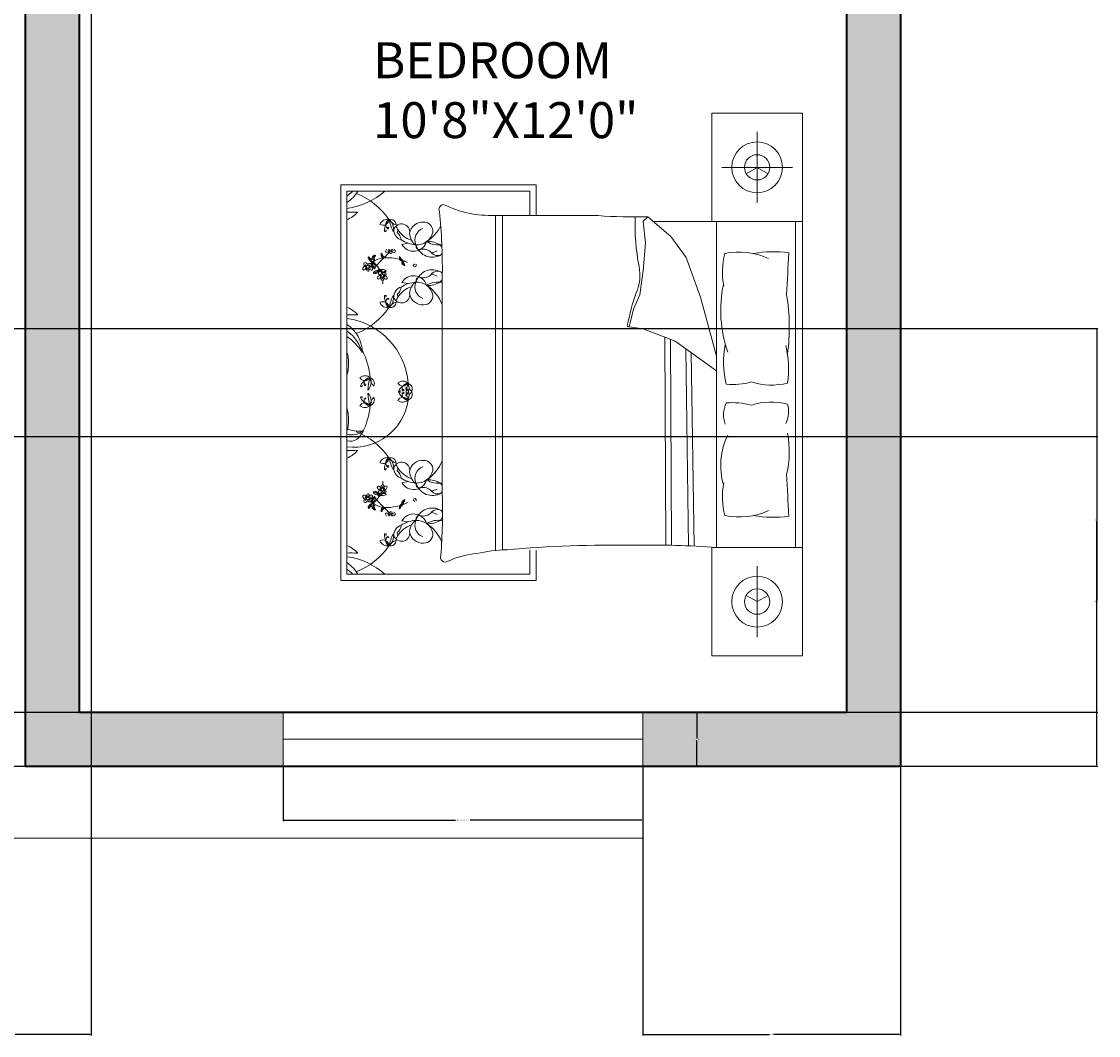
# Model space of a CAD drawing. Units: inches. Extents: x 37 to 706, y -568 to 110.
# Tile 16 of 24: x 526 to 706, y -568 to -398. Entities that reach past the tile are written whole.
import ezdxf

# ---------------------------------------------------------------- set-up
doc = ezdxf.new("R2010")
doc.units = ezdxf.units.IN
doc.header["$MEASUREMENT"] = 0
for name, color, linetype, lineweight in [('A-ANNO-DIMS', 2, 'Continuous', 18), ('A-AREA-IDEN', 7, 'Continuous', 18), ('A-FLOR-STRS', 7, 'Continuous', 18), ('A-FURN', 8, 'Continuous', 13), ('A-GLAZ', 4, 'Continuous', 18), ('A-WALL', 7, 'Continuous', 35), ('A-WALL-PATT', 252, 'Continuous', 13)]:
    doc.layers.add(name, color=color, linetype=linetype, lineweight=lineweight)
doc.styles.get("Standard").update_dxf_attribs({"font": 'arial.ttf'})
doc.dimstyles.get("Standard").update_dxf_attribs({"dimtxt": 0.18, "dimasz": 0.18, "dimexe": 0.18, "dimexo": 0.0625, "dimgap": 0.09, "dimtad": 0, "dimtih": 1, "dimtoh": 1, "dimdec": 0, "dimzin": 0, "dimdsep": 46, "dimlunit": 3, "dimtxsty": 'Standard', "dimcen": 0.09, "dimadec": 0, "dimazin": 0, "dimtfac": 1, "dimtdec": 0, "dimtofl": 0, "dimtmove": 0, "dimatfit": 3, "dimfxl": 1, "dimtolj": 1, "dimtzin": 0, "dimarcsym": 0})

# ---------------------------------------------------------------- blocks, each defined once
blk = doc.blocks.new('BED-DOUBLE-WITH-NIGHTSTANDS')
for p, q in [((77.02, 90.57), (77.02, 0)), ((69.47, 75.59), (69.47, 87.43)), ((63.56, 81.51), (75.39, 81.51)), ((0, 78.61), (32.62, 78.61)), ((0, 12.59), (0, 78.61)), ((1.05, 77.56), (1.05, 13.64)), ((31.58, 77.56), (1.05, 77.56)), ((31.58, 73.49), (31.58, 77.56)), ((32.62, 78.61), (32.62, 73.49)), ((25.85, 17.62), (25.85, 73.5)), ((26.98, 17.7), (26.98, 73.5)), ((50.48, 72.53), (51.22, 73.26)), ((50.85, 68.86), (50.48, 72.53)), ((51.22, 73.26), (55.07, 69.96)), ((77.02, 72.45), (52.16, 72.45)), ((62.71, 72.45), (62.71, 18.11)), ((75.86, 18.11), (75.86, 72.45)), ((10.23, 68.64), (11.25, 68.84)), ((50.48, 64.28), (50.85, 68.86)), ((55.07, 69.96), (57.63, 66.48)), ((57.63, 66.48), (60.02, 59.87)), ((16.95, 26.9), (16.95, 63.67)), ((49.93, 60.24), (50.48, 64.28)), ((10.23, 62.31), (11.25, 62.11)), ((48.83, 57.86), (49.93, 60.24)), ((60.02, 59.87), (62.71, 50)), ((48.1, 54.92), (48.83, 57.86)), ((50.48, 54.55), (48.1, 54.92)), ((55.8, 52.54), (50.48, 54.55)), ((54.24, 18.43), (54.09, 53.18)), ((55.17, 18.44), (55.03, 52.83)), ((62.71, 47.57), (55.8, 52.54)), ((58.02, 18.39), (57.55, 51.28)), ((58.95, 18.36), (58.49, 50.6)), ((10.23, 28.89), (11.25, 29.09)), ((10.23, 22.56), (11.25, 22.36)), ((31.58, 13.64), (31.58, 17.63)), ((32.62, 17.61), (32.62, 12.59)), ((69.47, 14.97), (69.47, 3.14)), ((32.62, 12.59), (0, 12.59)), ((1.05, 13.64), (31.58, 13.64))]:
    blk.add_line(p, q)
for points in [[(61.93, 72.45), (61.93, 90.57), (77.02, 90.57)], [(69.47, 81.51), (67.64, 80.45)], [(69.47, 81.51), (71.3, 80.45)], [(77.02, 18.11), (61.93, 18.11), (61.93, 0), (77.02, 0)], [(69.47, 9.06), (67.64, 10.11)], [(69.47, 9.06), (71.3, 10.11)]]:
    blk.add_lwpolyline(points)
for points in [[(42.92, 73.45, 0.001242), (25.74, 73.5, -0.127202), (17.18, 75.31)], [(74.76, 67.25, 0.074897), (68.85, 67.14, -0.472817)], [(68.52, 45.71, 0.14099), (74.55, 45.53, 0.235245)], [(68.52, 41.84, -0.14099), (74.55, 42.02, -0.235245)], [(74.76, 23.32, -0.074897), (68.85, 23.42, 0.472817)], [(27.69, 17.73, 0.056112), (22.71, 17.07, 0.095341), (17.91, 15.8)]]:
    blk.add_lwpolyline(points, format="xyb")
for centre, radius in [((69.47, 81.51), 4.23), ((69.47, 81.51), 2.11), ((4.52, 64.91), 0.231), ((6.95, 63.41), 0.231), ((6.95, 27.79), 0.231), ((4.52, 26.28), 0.231), ((69.47, 9.06), 4.23), ((69.47, 9.06), 2.11)]:
    blk.add_circle(centre, radius)
for centre, radius, start, end in [((-3.2, 82.51), 7.18, 306.3036, 316.4814), ((-2.13, 80.43), 5.76, 303.4617, 330.1116), ((-0.54, 86.37), 11.83, 277.745, 311.8856), ((-1.71, 66.13), 11.83, 34.3865, 68.5908), ((-0.79, 77.21), 4.81, 292.5547, 318.9546), ((1.79, 90.38), 16.36, 267.4081, 273.6519), ((17.23, 74.48), 0.836, 93.98, 207.3412), ((-77.32, 64.75), 94.28, 359.3433, 5.6887), ((7.77, 71.53), 1.31, 77.7115, 159.0387), ((7.06, 72.84), 0.988, 238.4633, 358.2869), ((10.3, 70.85), 2.99, 138.8402, 177.9352), ((8.5, 71.96), 0.967, 117.6827, 223.7762), ((8.28, 71.86), 0.98, 2.9516, 103.728), ((16.12, 74.61), 8.27, 192.5173, 207.1824), ((6.95, 71.3), 1.87, 345.4653, 54.2343), ((9.77, 73.87), 2.02, 211.3827, 255.2969), ((10.16, 70.71), 1.36, 350.264, 160.8688), ((13.65, 70.21), 2.16, 84.9449, 172.8857), ((13.86, 70.84), 1.53, 354.4856, 91.0538), ((48.97, 156.3), 83.07, 265.8294, 271.553), ((83.29, 71.71), 34.18, 177.4519, 191.3392), ((7.46, 70.95), 0.147, 177.9352, 11.4834), ((7.53, 70.96), 0.0713, 11.4834, 127.9409), ((7.89, 71.38), 0.128, 223.7762, 159.7183), ((10.57, 71.04), 1.7, 175.969, 254.3045), ((8.69, 70.99), 0.833, 333.9755, 53.2681), ((8.31, 69.21), 1.81, 6.1662, 51.5825), ((13.15, 73.4), 4.28, 211.2614, 251.7045), ((14.13, 70.59), 2.63, 182.3591, 234.0401), ((14.47, 69.36), 2.1, 111.5819, 201.4221), ((12.73, 71.31), 2.72, 265.2933, 346.921), ((10.57, 74.83), 6.85, 303.6671, 333.2997), ((12.81, 73.44), 4.86, 236.2883, 266.5076), ((12.18, 69.76), 2.25, 209.9085, 343.1337), ((13.13, 68.34), 0.562, 167.3041, 285.1471), ((14.65, 65.65), 3.49, 122.7011, 126.3445), ((15.31, 69.41), 2.89, 199.2822, 299.1751), ((16.28, 72.32), 3.75, 238.8218, 279.1554), ((14.65, 65.65), 3.49, 55.785, 94.7304), ((15.95, 67.67), 1.09, 30.0293, 52.325), ((4.85, 66.4), 0.258, 124.3538, 214.3923), ((5.41, 66.58), 0.697, 176.9701, 248.2913), ((10.38, 70.25), 6.74, 212.6784, 216.3746), ((5.81, 66.23), 0.6, 122.8155, 187.3992), ((6.07, 66.15), 0.697, 109.4799, 177.6828), ((5.7, 66.59), 0.258, 56.8636, 146.9021), ((11.37, 62.96), 6.74, 145.1882, 148.8844), ((9.29, 67.11), 2.55, 178.3264, 187.1302), ((6.53, 66.75), 0.476, 11.3256, 64.4621), ((8.15, 67.44), 1.43, 190.2588, 210.656), ((7.19, 66.85), 0.435, 188.3432, 274.2869), ((7.57, 67.09), 0.759, 210.656, 242.6341), ((8.14, 67.75), 1.46, 218.2101, 226.3071), ((7.07, 66.52), 0.185, 325.7657, 67.4417), ((1.34, 72.69), 8.6, 313.1541, 322.0459), ((7.66, 67.53), 0.177, 142.4737, 265.053), ((7.89, 67.56), 0.381, 127.7621, 169.0403), ((7.69, 67.89), 0.536, 265.053, 338.3618), ((8.4, 67.15), 0.7, 113.4276, 137.6104), ((8.32, 67.88), 0.231, 183.2768, 356.7232), ((8.49, 67.46), 0.377, 139.7889, 227.6792), ((8.37, 67.33), 0.199, 227.6792, 350.3487), ((7.6, 67.46), 0.755, 353.0852, 15.7171), ((8.1, 67.37), 0.477, 350.3487, 43.6538), ((8.98, 67.87), 0.555, 198.7263, 262.5032), ((8.54, 67.61), 0.22, 1.1081, 91.8675), ((8.68, 67.56), 0.385, 11.5637, 52.6358), ((8.95, 67.49), 0.178, 255.2356, 54.9248), ((12.34, 66.57), 2.55, 178.3264, 187.1302), ((9.58, 66.21), 0.476, 11.3256, 64.4621), ((11.19, 66.9), 1.43, 190.2588, 210.656), ((13.76, 66), 1.86, 41.5653, 105.1471), ((14.78, 69.85), 2.6, 277.436, 299.9149), ((16.16, 68.13), 1.36, 221.5653, 293.8354), ((15.95, 67.67), 1.09, 314.4517, 333.558), ((75.82, 64.02), 12.14, 165.1039, 191.0369), ((66.47, 55.71), 11.67, 65.1316, 101.7583), ((936.66, 17.33), 863.34, 176.68521, 177.14978), ((3.86, 64.56), 0.177, 142.4737, 265.053), ((4.09, 64.6), 0.381, 61.2196, 169.0403), ((3.89, 64.92), 0.536, 265.053, 338.3618), ((4.34, 65.38), 0.455, 157.4086, 261.4386), ((4.09, 65.4), 0.229, 58.0499, 135.6268), ((4.6, 64.19), 0.7, 113.4276, 137.6104), ((4.32, 65.26), 0.153, 172.906, 277.132), ((3.82, 64.98), 0.727, 14.7558, 58.0499), ((4.69, 64.5), 0.377, 139.7889, 227.6792), ((4.84, 65.17), 0.315, 36.1046, 181.4281), ((3.8, 64.5), 0.755, 353.0852, 15.7171), ((5.23, 66.36), 0.6, 190.3057, 287.1958), ((4.29, 64.41), 0.477, 350.3487, 43.6538), ((5.18, 64.9), 0.555, 198.7263, 262.5032), ((4.66, 65.42), 0.317, 270.0645, 331.1507), ((4.93, 65.34), 0.363, 221.8413, 265.7877), ((4.74, 64.65), 0.22, 1.1081, 91.8675), ((4.92, 65.2), 0.226, 263.7526, 41.7054), ((4.88, 64.6), 0.385, 11.5637, 86.365), ((5.17, 66.41), 0.267, 216.3746, 291.7548), ((7.53, 62.67), 3.76, 124.0033, 132.4917), ((5.15, 64.53), 0.178, 255.2356, 54.9248), ((3.66, 62.2), 4.02, 63.7819, 68.2913), ((5.81, 65.29), 0.639, 128.3208, 208.8162), ((5.92, 65.34), 0.764, 207.7043, 254.3516), ((5.34, 65.98), 0.201, 289.3605, 111.7548), ((5.49, 65.98), 0.201, 221.8703, 44.2646), ((6.41, 65.39), 1.05, 157.2305, 229.0635), ((6.05, 65.74), 0.619, 174.4544, 220.6188), ((2.53, 62.29), 4.51, 30.544, 49.818), ((5.83, 66.31), 0.267, 148.8844, 224.2646), ((5.02, 64.86), 0.744, 340.0041, 40.6188), ((7.53, 62.67), 3.76, 94.756, 119.2041), ((15.54, 57.26), 12.37, 132.2412, 142.1744), ((7.72, 58.94), 7.5, 73.5842, 93.8277), ((10.23, 66.31), 0.435, 188.3432, 274.2869), ((10.61, 66.55), 0.759, 210.656, 242.6341), ((11.19, 67.21), 1.46, 218.2101, 226.3071), ((10.11, 65.98), 0.185, 325.7657, 67.4417), ((10.63, 65.65), 0.435, 147.5332, 233.4768), ((11.02, 65.87), 0.759, 179.1859, 211.164), ((10.28, 65.7), 0.185, 354.3784, 96.0543), ((7.72, 58.94), 7.5, 63.0032, 69.8941), ((11.6, 66.22), 1.43, 211.164, 231.5612), ((11.85, 67.38), 2.55, 234.6898, 243.4936), ((11.87, 66.07), 1.46, 195.5129, 203.6099), ((10.23, 65.12), 0.476, 357.3579, 50.4944), ((12.28, 65.21), 0.175, 12.7051, 190.4384), ((12.38, 65.23), 0.284, 190.4384, 10.4136), ((42.55, 63.54), 7.37, 336.2616, 11.3392), ((4.57, 64.37), 0.199, 227.6792, 350.3487), ((5.43, 64.9), 1.05, 270.278, 342.111), ((6.13, 63.58), 0.744, 98.7227, 159.3375), ((5.75, 64.54), 0.764, 244.9899, 291.6373), ((5.92, 64.93), 0.619, 278.7227, 324.8872), ((5.81, 64.43), 0.639, 290.5253, 358.5375), ((6.29, 63.06), 0.177, 142.4737, 265.053), ((6.52, 63.09), 0.381, 61.2196, 169.0403), ((6.32, 63.41), 0.536, 265.053, 338.3618), ((6.77, 63.88), 0.455, 157.4086, 261.4386), ((6.52, 63.89), 0.229, 58.0499, 135.6268), ((7.06, 64.61), 0.639, 182.8499, 266.1226), ((6.81, 65.06), 0.619, 231.7607, 277.9252), ((7.29, 65.17), 1.05, 214.5369, 286.3699), ((7.03, 62.68), 0.7, 113.4276, 137.6104), ((6.76, 63.75), 0.153, 172.906, 277.132), ((6.25, 63.47), 0.727, 14.7558, 58.0499), ((2.53, 62.29), 4.51, 23.0501, 23.8477), ((7.12, 62.99), 0.377, 139.7889, 227.6792), ((7, 63.71), 0.744, 37.3105, 97.9252), ((7.27, 63.66), 0.315, 36.1046, 181.4281), ((6.23, 62.99), 0.755, 353.0852, 15.7171), ((7.08, 64.73), 0.764, 265.0106, 311.658), ((6.72, 62.9), 0.477, 350.3487, 43.6538), ((7.61, 63.4), 0.555, 198.7263, 262.5032), ((7.09, 63.91), 0.317, 270.0645, 331.1507), ((7.36, 63.83), 0.363, 221.8413, 265.7877), ((7.17, 63.14), 0.22, 1.1081, 91.8675), ((7.36, 63.7), 0.226, 263.7526, 41.7054), ((7.31, 63.09), 0.385, 11.5637, 86.365), ((7.58, 63.02), 0.178, 255.2356, 54.9248), ((12.18, 61.19), 2.25, 16.8663, 150.0915), ((13.13, 62.61), 0.562, 74.8529, 192.6959), ((15.31, 61.54), 2.89, 60.8249, 160.7178), ((13.76, 64.95), 1.86, 254.8529, 318.4347), ((14.78, 61.1), 2.6, 60.0851, 82.564), ((16.16, 62.82), 1.36, 66.1646, 138.4347), ((15.95, 63.28), 1.09, 23.229, 45.5483), ((7, 62.86), 0.199, 227.6792, 350.3487), ((2.53, 62.29), 4.51, 357.1071, 4.7585), ((10.57, 59.91), 1.7, 105.6955, 184.031), ((8.31, 61.74), 1.81, 308.4175, 353.8338), ((13.15, 57.54), 4.28, 108.2955, 148.7386), ((12.81, 57.5), 4.86, 93.4924, 123.7117), ((14.13, 60.36), 2.63, 125.9599, 177.6409), ((14.47, 61.59), 2.1, 158.5779, 248.4181), ((12.73, 59.64), 2.72, 13.079, 94.7067), ((14.65, 65.3), 3.49, 233.6555, 237.2989), ((16.28, 58.63), 3.75, 79.7133, 121.1782), ((14.65, 65.3), 3.49, 265.2696, 304.215), ((10.57, 56.11), 6.85, 21.4941, 56.3329), ((15.95, 63.28), 1.09, 307.675, 336.7144), ((84.45, 57.63), 21.05, 168.0397, 199.2615), ((7.46, 60), 0.147, 348.5166, 182.0648), ((10.3, 60.1), 2.99, 182.0648, 221.1598), ((7.53, 59.98), 0.0713, 232.0591, 348.5166), ((8.5, 58.99), 0.967, 136.2238, 242.3173), ((7.94, 59.56), 0.0771, 200.2667, 136.2271), ((6.95, 59.65), 1.87, 305.7657, 14.5347), ((16.12, 56.34), 8.27, 152.8176, 167.4827), ((10.16, 60.24), 1.36, 199.1312, 9.736), ((8.69, 59.96), 0.833, 306.7319, 26.0245), ((13.65, 60.74), 2.16, 187.1143, 275.0551), ((13.86, 60.11), 1.53, 268.9462, 5.5144), ((82.33, 48.63), 35.12, 160.1194, 169.3383), ((41.99, 54.84), 32.85, 352.2196, 9.497), ((-0.79, 53.74), 4.81, 41.0454, 67.4453), ((-1.71, 64.81), 11.83, 291.4092, 325.6135), ((7.06, 58.1), 0.988, 1.7131, 121.5367), ((7.77, 59.41), 1.31, 200.9613, 282.2885), ((8.28, 59.09), 0.98, 256.272, 357.0484), ((9.77, 57.08), 2.02, 104.7031, 148.6173), ((1.79, 40.57), 16.36, 86.3481, 92.5919), ((-0.54, 44.58), 11.83, 4.4623, 82.255), ((-2.13, 50.51), 5.76, 1.272, 56.5383), ((-3.2, 48.44), 7.18, 17.8504, 53.6964), ((48.03, 55.13), 0.219, 178.8623, 289.7536), ((-5.22, 44.66), 10.68, 34.0123, 54.053), ((-5.17, 48.79), 6.5, 343.5431, 17.0202), ((-6.88, 45.48), 11.83, 4.4623, 27.4146), ((79.85, 49.11), 15.97, 169.8617, 193.6238), ((58.59, 47.9), 16.14, 351.5249, 13.96), ((-8.52, 46.22), 9.62, 4.3787, 5.6357), ((-15.11, 41.15), 17.18, 19.7217, 19.9028), ((4.03, 45.43), 1.31, 47.7873, 129.1145), ((4.07, 46.92), 0.988, 208.5391, 328.3627), ((3.47, 45.08), 0.147, 148.011, 341.5592), ((5.88, 43.58), 2.99, 108.9159, 148.011), ((3.54, 45.06), 0.0713, 341.5592, 98.0167), ((4.87, 45.44), 0.967, 87.7585, 193.852), ((4.06, 45.24), 0.128, 193.852, 129.9245), ((12.81, 43.93), 8.27, 162.593, 177.2582), ((3.21, 45.64), 1.87, 315.5411, 24.3101), ((6.93, 46.46), 2.02, 181.4585, 225.3727), ((4.64, 45.46), 0.98, 333.0274, 73.8037), ((10.37, 44.53), 1.31, 47.7873, 129.1145), ((10.41, 46.02), 0.988, 208.5391, 328.3627), ((12.22, 42.67), 2.99, 108.9159, 148.011), ((11.21, 44.53), 0.967, 87.7585, 193.852), ((9.54, 44.73), 1.87, 315.5411, 24.3101), ((19.14, 43.02), 8.27, 162.593, 177.2582), ((10.97, 44.56), 0.98, 333.0274, 73.8037), ((13.27, 45.55), 2.02, 181.4585, 225.3727), ((65.49, 56.38), 11.1, 264.0129, 285.8293), ((3.47, 43.1), 0.147, 18.4408, 211.989), ((3.54, 43.12), 0.0713, 261.9833, 18.4408), ((12.81, 44.25), 8.27, 182.7418, 197.407), ((3.21, 42.54), 1.87, 335.6899, 44.4589), ((6.93, 41.72), 2.02, 134.6273, 178.5415), ((4.64, 42.72), 0.98, 286.1963, 26.9726), ((10.41, 42.16), 0.988, 31.6373, 151.4609), ((9.8, 44.18), 0.147, 148.011, 341.5592), ((9.8, 44), 0.147, 18.4408, 211.989), ((12.22, 45.51), 2.99, 211.989, 251.0841), ((9.88, 44.15), 0.0713, 341.5592, 98.0167), ((9.88, 44.03), 0.0713, 261.9833, 18.4408), ((11.21, 43.65), 0.967, 166.148, 272.2415), ((10.39, 44.33), 0.128, 193.852, 129.9245), ((10.44, 43.86), 0.0771, 230.1909, 166.0209), ((9.54, 43.45), 1.87, 335.6899, 44.4589), ((19.14, 45.16), 8.27, 182.7418, 197.407), ((10.97, 43.62), 0.98, 286.1963, 26.9726), ((13.27, 42.63), 2.02, 134.6273, 178.5415), ((2.19, 43.98), 9.15, 262.8636, 351.8197), ((4.07, 41.26), 0.988, 31.6373, 151.4609), ((4.03, 42.75), 1.31, 230.8855, 312.2127), ((5.88, 44.6), 2.99, 211.989, 251.0841), ((-6.88, 42.69), 11.83, 332.5854, 355.5377), ((4.87, 42.74), 0.967, 166.148, 272.2415), ((4.11, 42.95), 0.0771, 230.1909, 166.0209), ((10.37, 43.65), 1.31, 230.8855, 312.2127), ((68.68, 40.17), 4.8, 155.0183, 198.5407), ((65.49, 31.16), 11.1, 74.1707, 95.9871), ((70.25, 40.78), 4.48, 333.3437, 16.1026), ((-5.17, 39.39), 6.5, 342.9798, 16.4569), ((-8.52, 41.96), 9.62, 354.3643, 355.6213), ((-15.11, 47.03), 17.18, 340.0972, 340.2783), ((3.02, 42.8), 5.3, 248.117, 276.6195), ((1.55, 37.94), 2.12, 256.3898, 349.0739), ((1.84, 39.54), 2.68, 252.8609, 311.9049), ((-1.71, 26.39), 11.83, 34.3865, 68.5908), ((74.93, 31.78), 11.53, 153.8761, 196.1746), ((58.92, 34.06), 15.92, 346.3427, 11.1841), ((1.79, 50.63), 16.36, 267.4081, 273.6519), ((-0.79, 37.46), 4.81, 292.5547, 318.9546), ((7.77, 31.78), 1.31, 77.7115, 159.0387), ((7.06, 33.09), 0.988, 238.4633, 358.2869), ((10.3, 31.1), 2.99, 138.8402, 177.9352), ((8.5, 32.21), 0.967, 117.6827, 223.7762), ((8.28, 32.11), 0.98, 2.9516, 103.728), ((9.77, 34.12), 2.02, 211.3827, 255.2969), ((6.95, 31.55), 1.87, 345.4653, 54.2343), ((16.12, 34.86), 8.27, 192.5173, 207.1824), ((13.65, 30.46), 2.16, 84.9449, 172.8857), ((13.86, 31.09), 1.53, 354.4856, 91.0538), ((10.57, 35.08), 6.85, 303.6671, 338.5059), ((7.46, 31.2), 0.147, 177.9352, 11.4834), ((7.53, 31.21), 0.0713, 11.4834, 127.9409), ((7.89, 31.63), 0.128, 223.7762, 159.7183), ((10.16, 30.96), 1.36, 350.264, 160.8688), ((10.57, 31.29), 1.7, 175.969, 254.3045), ((8.69, 31.24), 0.833, 333.9755, 53.2681), ((8.31, 29.46), 1.81, 6.1662, 51.5825), ((13.15, 33.66), 4.28, 211.2614, 251.7045), ((14.13, 30.84), 2.63, 182.3591, 234.0401), ((14.47, 29.61), 2.1, 111.5819, 201.4221), ((12.73, 31.56), 2.72, 265.2933, 346.921), ((2.53, 28.91), 4.51, 355.2415, 2.8929), ((12.81, 33.7), 4.86, 236.2883, 266.5076), ((12.18, 30.01), 2.25, 209.9085, 343.1337), ((14.65, 25.9), 3.49, 122.7011, 126.3445), ((16.28, 32.57), 3.75, 238.8218, 280.2867), ((14.65, 25.9), 3.49, 55.785, 94.7304), ((15.95, 27.92), 1.09, 23.2856, 52.325), ((75.82, 26.55), 12.14, 168.9631, 194.8961), ((936.66, 73.23), 863.34, 182.85022, 183.31479), ((4.69, 26.7), 0.377, 132.3208, 220.2111), ((4.57, 26.83), 0.199, 9.6513, 132.3208), ((5.75, 26.66), 0.764, 68.3627, 115.0101), ((5.43, 26.3), 1.05, 17.889, 89.722), ((6.13, 27.61), 0.744, 200.6625, 261.2773), ((5.81, 26.77), 0.639, 1.4625, 69.4747), ((6.29, 28.14), 0.177, 94.947, 217.5263), ((6.52, 28.11), 0.381, 190.9597, 298.7804), ((6.32, 27.78), 0.536, 21.6382, 94.947), ((6.77, 27.32), 0.455, 98.5614, 202.5914), ((6.52, 27.31), 0.229, 224.3732, 301.9501), ((7.06, 26.59), 0.639, 93.8774, 177.1501), ((7.29, 26.03), 1.05, 73.6301, 145.4631), ((7.03, 28.52), 0.7, 222.3896, 246.5724), ((6.76, 27.45), 0.153, 82.868, 187.094), ((6.25, 27.73), 0.727, 301.9501, 345.2442), ((2.53, 28.91), 4.51, 336.1523, 336.9499), ((7.12, 28.21), 0.377, 132.3208, 220.2111), ((7, 28.34), 0.199, 9.6513, 132.3208), ((7, 27.49), 0.744, 262.0748, 322.6895), ((6.23, 28.2), 0.755, 344.2829, 6.9148), ((7.27, 27.54), 0.315, 178.5719, 323.8954), ((7.08, 26.46), 0.764, 48.342, 94.9894), ((6.72, 28.3), 0.477, 316.3462, 9.6513), ((7.61, 27.8), 0.555, 97.4968, 161.2737), ((7.36, 27.37), 0.363, 94.2123, 138.1587), ((7.09, 27.29), 0.317, 28.8493, 89.9355), ((7.17, 28.06), 0.22, 268.1325, 358.8919), ((7.31, 28.11), 0.385, 273.635, 348.4363), ((7.36, 27.5), 0.226, 318.2946, 96.2474), ((7.58, 28.18), 0.178, 305.0752, 104.7644), ((13.13, 28.59), 0.562, 167.3041, 285.1471), ((15.31, 29.66), 2.89, 199.2822, 299.1751), ((13.76, 26.25), 1.86, 41.5653, 105.1471), ((14.78, 30.1), 2.6, 277.436, 299.9149), ((16.16, 28.38), 1.36, 221.5653, 293.8354), ((15.95, 27.92), 1.09, 314.4517, 336.7144), ((3.86, 26.63), 0.177, 94.947, 217.5263), ((4.09, 26.6), 0.381, 190.9597, 298.7804), ((3.89, 26.28), 0.536, 21.6382, 94.947), ((4.34, 25.81), 0.455, 98.5614, 202.5914), ((4.09, 25.8), 0.229, 224.3732, 301.9501), ((4.6, 27.01), 0.7, 222.3896, 246.5724), ((4.32, 25.94), 0.153, 82.868, 187.094), ((3.82, 26.22), 0.727, 301.9501, 345.2442), ((4.84, 26.03), 0.315, 178.5719, 323.8954), ((3.8, 26.7), 0.755, 344.2829, 6.9148), ((4.29, 26.79), 0.477, 316.3462, 9.6513), ((5.23, 24.83), 0.6, 72.8042, 169.6943), ((5.18, 26.29), 0.555, 97.4968, 161.2737), ((4.93, 25.86), 0.363, 94.2123, 138.1587), ((4.66, 25.78), 0.317, 28.8493, 89.9355), ((5.41, 24.62), 0.697, 111.7087, 183.0299), ((4.74, 26.55), 0.22, 268.1325, 358.8919), ((4.88, 26.6), 0.385, 273.635, 348.4363), ((4.92, 25.99), 0.226, 318.2946, 96.2474), ((7.53, 28.53), 3.76, 227.5083, 235.9967), ((5.15, 26.67), 0.178, 305.0752, 104.7644), ((3.66, 29), 4.02, 291.7087, 296.2181), ((5.81, 25.91), 0.639, 151.1838, 231.6792), ((5.92, 25.86), 0.764, 105.6484, 152.2957), ((5.34, 25.22), 0.201, 248.2452, 70.6395), ((6.41, 25.8), 1.05, 130.9365, 202.7695), ((5.49, 25.22), 0.201, 315.7354, 138.1297), ((6.05, 25.46), 0.619, 139.3812, 185.5456), ((2.53, 28.91), 4.51, 310.182, 329.456), ((5.02, 26.34), 0.744, 319.3812, 19.9959), ((7.53, 28.53), 3.76, 240.7959, 265.244), ((15.54, 33.94), 12.37, 217.8256, 227.7588), ((5.92, 26.27), 0.619, 35.1128, 81.2773), ((6.81, 26.14), 0.619, 82.0748, 128.2393), ((10.23, 24.88), 0.435, 85.7131, 171.6568), ((10.61, 24.64), 0.759, 117.3659, 149.344), ((10.11, 25.21), 0.185, 292.5583, 34.2343), ((10.63, 25.55), 0.435, 126.5232, 212.4668), ((11.02, 25.33), 0.759, 148.836, 180.8141), ((10.28, 25.5), 0.185, 263.9457, 5.6216), ((7.72, 32.26), 7.5, 290.1059, 296.9968), ((11.6, 24.98), 1.43, 128.4388, 148.836), ((11.85, 23.82), 2.55, 116.5064, 125.3102), ((11.87, 25.13), 1.46, 156.3901, 164.4871), ((10.23, 26.08), 0.476, 309.5056, 2.6421), ((12.28, 25.98), 0.175, 169.5616, 347.2949), ((12.38, 25.96), 0.284, 349.5864, 169.5616), ((-71.13, 24.12), 88.13, 355.2402, 1.8035), ((4.85, 24.8), 0.258, 145.6077, 235.6462), ((10.38, 20.95), 6.74, 143.6254, 147.3216), ((5.17, 24.78), 0.267, 68.2452, 143.6254), ((5.81, 24.97), 0.6, 172.6008, 237.1845), ((6.07, 25.05), 0.697, 182.3172, 250.5201), ((5.7, 24.61), 0.258, 213.0979, 303.1364), ((5.83, 24.89), 0.267, 135.7354, 211.1156), ((11.37, 28.24), 6.74, 211.1156, 214.8118), ((8.15, 23.76), 1.43, 149.344, 169.7412), ((9.29, 24.09), 2.55, 172.8698, 181.6736), ((6.53, 24.45), 0.476, 295.5379, 348.6744), ((7.19, 24.34), 0.435, 85.7131, 171.6568), ((7.57, 24.1), 0.759, 117.3659, 149.344), ((8.14, 23.45), 1.46, 133.6929, 141.7899), ((7.07, 24.67), 0.185, 292.5583, 34.2343), ((7.72, 32.26), 7.5, 266.1723, 286.4158), ((1.34, 18.5), 8.6, 37.9541, 46.8459), ((7.66, 23.67), 0.177, 94.947, 217.5263), ((7.89, 23.64), 0.381, 190.9597, 232.2379), ((7.69, 23.31), 0.536, 21.6382, 94.947), ((8.4, 24.05), 0.7, 222.3896, 246.5724), ((8.32, 23.32), 0.231, 3.2768, 176.7232), ((8.49, 23.74), 0.377, 132.3208, 220.2111), ((8.37, 23.87), 0.199, 9.6513, 132.3208), ((7.6, 23.73), 0.755, 344.2829, 6.9148), ((8.1, 23.82), 0.477, 316.3462, 9.6513), ((8.98, 23.33), 0.555, 97.4968, 161.2737), ((8.54, 23.59), 0.22, 268.1325, 358.8919), ((8.95, 23.71), 0.178, 305.0752, 104.7644), ((8.68, 23.64), 0.385, 307.3642, 348.4363), ((11.19, 24.3), 1.43, 149.344, 169.7412), ((12.34, 24.63), 2.55, 172.8698, 181.6736), ((9.58, 24.98), 0.476, 295.5379, 348.6744), ((11.19, 23.99), 1.46, 133.6929, 141.7899), ((12.18, 21.44), 2.25, 16.8663, 150.0915), ((13.13, 22.86), 0.562, 74.8529, 192.6959), ((15.31, 21.79), 2.89, 60.8249, 160.7178), ((13.76, 25.2), 1.86, 254.8529, 318.4347), ((14.78, 21.35), 2.6, 60.0851, 82.564), ((16.16, 23.07), 1.36, 66.1646, 138.4347), ((15.95, 23.53), 1.09, 16.6343, 45.5483), ((66.47, 34.85), 11.67, 258.2417, 294.8684), ((10.57, 20.16), 1.7, 105.6955, 184.031), ((8.31, 21.99), 1.81, 308.4175, 353.8338), ((13.15, 17.79), 4.28, 108.2955, 148.7386), ((12.81, 17.75), 4.86, 93.4924, 123.7117), ((14.13, 20.61), 2.63, 125.9599, 177.6409), ((14.47, 21.84), 2.1, 158.5779, 248.4181), ((12.73, 19.89), 2.72, 13.079, 94.7067), ((14.65, 25.55), 3.49, 233.6555, 237.2989), ((16.28, 18.88), 3.75, 79.249, 121.1782), ((14.65, 25.55), 3.49, 265.2696, 304.215), ((10.57, 16.37), 6.85, 23.6453, 56.3329), ((15.95, 23.53), 1.09, 307.675, 342.5814), ((7.46, 20.25), 0.147, 348.5166, 182.0648), ((10.3, 20.35), 2.99, 182.0648, 221.1598), ((7.53, 20.24), 0.0713, 232.0591, 348.5166), ((8.5, 19.24), 0.967, 136.2238, 242.3173), ((7.94, 19.81), 0.0771, 200.2667, 136.2271), ((16.12, 16.59), 8.27, 152.8176, 167.4827), ((6.95, 19.9), 1.87, 305.7657, 14.5347), ((10.16, 20.49), 1.36, 199.1312, 9.736), ((8.69, 20.21), 0.833, 306.7319, 26.0245), ((13.65, 20.99), 2.16, 187.1143, 275.0551), ((13.86, 20.36), 1.53, 268.9462, 5.5144), ((-0.79, 13.99), 4.81, 41.0454, 67.4453), ((-1.71, 25.06), 11.83, 291.4092, 325.6135), ((7.06, 18.36), 0.988, 1.7131, 121.5367), ((7.77, 19.67), 1.31, 200.9613, 282.2885), ((9.77, 17.33), 2.02, 104.7031, 148.6173), ((8.28, 19.34), 0.98, 256.272, 357.0484), ((45.72, -193.78), 212.28, 89.1145, 94.8735), ((51.64, -144.24), 162.73, 86.1, 90.9282), ((1.79, 0.82), 16.36, 86.3481, 92.5919), ((-0.54, 4.83), 11.83, 48.1144, 82.255), ((17.45, 16.48), 0.826, 156.5219, 303.8264), ((-2.13, 10.76), 5.76, 29.8884, 56.5383), ((-3.2, 8.69), 7.18, 43.5186, 53.6964)]:
    blk.add_arc(centre, radius, start, end)
blk = doc.blocks.new('WIN-60')
for p, q in [((60, 9), (0, 9)), ((0, 9), (0, 0)), ((60, 0), (60, 9)), ((60, 4.5), (0, 4.5)), ((0, 0), (60, 0))]:
    blk.add_line(p, q)
blk = doc.blocks.new('ENTRY-STEP-236')
for p, q in [((236, 12), (236, 0)), ((236, 0), (0, 0))]:
    blk.add_line(p, q)
blk = doc.blocks.new('*D19')
at = {"layer": 'A-ANNO-DIMS', "color": 0, "lineweight": -2, "transparency": 16777216}
for p, q in [((569.96, -522.77), (569.96, -531.89)), ((629.96, -522.77), (629.96, -531.89)), ((570.14, -531.71), (598.73, -531.71)), ((629.78, -531.71), (601.19, -531.71))]:
    blk.add_line(p, q, dxfattribs=at)
at = {"layer": 'A-ANNO-DIMS', "color": 0, "transparency": 16777216}
for points in [[(570.14, -531.68), (570.14, -531.74), (569.96, -531.71)], [(629.78, -531.68), (629.78, -531.74), (629.96, -531.71)]]:
    blk.add_solid(points, dxfattribs=at)
at = {"layer": 'Defpoints', "color": 0, "transparency": 16777216}
for p in [(569.96, -522.71), (629.96, -522.71), (629.96, -531.71)]:
    blk.add_point(p, dxfattribs=at)
at = {"layer": 'A-ANNO-DIMS', "color": 0, "transparency": 16777216, "insert": (599.96, -531.71), "char_height": 0.18, "attachment_point": 5}
blk.add_mtext('\\A1;WINDOW 5\'-0" TYP.', dxfattribs=at)
blk = doc.blocks.new('*D20')
at = {"layer": 'A-ANNO-DIMS', "color": 0, "lineweight": -2, "transparency": 16777216}
for p, q in [((630.02, -513.71), (639.14, -513.71)), ((638.96, -513.89), (638.96, -518.03)), ((638.96, -522.53), (638.96, -518.39)), ((630.02, -522.71), (639.14, -522.71))]:
    blk.add_line(p, q, dxfattribs=at)
at = {"layer": 'A-ANNO-DIMS', "color": 0, "transparency": 16777216}
for points in [[(638.93, -513.89), (638.99, -513.89), (638.96, -513.71)], [(638.93, -522.53), (638.99, -522.53), (638.96, -522.71)]]:
    blk.add_solid(points, dxfattribs=at)
at = {"layer": 'Defpoints', "color": 0, "transparency": 16777216}
for p in [(629.96, -513.71), (638.96, -513.71), (629.96, -522.71)]:
    blk.add_point(p, dxfattribs=at)
at = {"layer": 'A-ANNO-DIMS', "color": 0, "transparency": 16777216, "insert": (638.96, -518.21), "char_height": 0.18, "attachment_point": 5}
blk.add_mtext('\\A1;0\'-9" TYP.', dxfattribs=at)
blk = doc.blocks.new('*D45')
at = {"layer": 'A-ANNO-DIMS', "color": 0, "lineweight": -2, "transparency": 16777216}
for p, q in [((88.02, -449.71), (705.89, -449.71)), ((705.71, -449.89), (705.71, -481.53)), ((705.71, -513.53), (705.71, -481.89)), ((79.02, -513.71), (705.89, -513.71))]:
    blk.add_line(p, q, dxfattribs=at)
at = {"layer": 'A-ANNO-DIMS', "color": 0, "transparency": 16777216}
for points in [[(705.68, -449.89), (705.74, -449.89), (705.71, -449.71)], [(705.68, -513.53), (705.74, -513.53), (705.71, -513.71)]]:
    blk.add_solid(points, dxfattribs=at)
at = {"layer": 'Defpoints', "color": 0, "transparency": 16777216}
for p in [(87.96, -449.71), (705.71, -449.71), (78.96, -513.71)]:
    blk.add_point(p, dxfattribs=at)
at = {"layer": 'A-ANNO-DIMS', "color": 0, "transparency": 16777216, "insert": (705.71, -481.71), "char_height": 0.18, "attachment_point": 5}
blk.add_mtext('\\A1;5\'-4"', dxfattribs=at)
blk = doc.blocks.new('*D46')
at = {"layer": 'A-ANNO-DIMS', "color": 0, "lineweight": -2, "transparency": 16777216}
for p, q in [((403.020833, -467.708464), (705.888333, -467.708464)), ((705.708333, -467.888464), (705.708333, -495.028464)), ((705.708333, -522.528464), (705.708333, -495.388464)), ((394.020833, -522.708464), (705.888333, -522.708464))]:
    blk.add_line(p, q, dxfattribs=at)
at = {"layer": 'A-ANNO-DIMS', "color": 0, "transparency": 16777216}
for points in [[(705.678333, -467.888464), (705.738333, -467.888464), (705.708333, -467.708464)], [(705.678333, -522.528464), (705.738333, -522.528464), (705.708333, -522.708464)]]:
    blk.add_solid(points, dxfattribs=at)
at = {"layer": 'Defpoints', "color": 0, "transparency": 16777216}
for p in [(402.958333, -467.708464), (705.708333, -467.708464), (393.958333, -522.708464)]:
    blk.add_point(p, dxfattribs=at)
at = {"layer": 'A-ANNO-DIMS', "color": 0, "transparency": 16777216, "insert": (705.708333, -495.208464), "char_height": 0.18, "attachment_point": 5}
blk.add_mtext('\\A1;4\'-7"', dxfattribs=at)
blk = doc.blocks.new('*D48')
at = {"layer": 'A-ANNO-DIMS', "color": 0, "lineweight": -2, "transparency": 16777216}
for p, q in [((629.96, -522.77), (629.96, -567.64)), ((672.96, -522.77), (672.96, -567.64)), ((630.14, -567.46), (651.13, -567.46)), ((672.78, -567.46), (651.79, -567.46))]:
    blk.add_line(p, q, dxfattribs=at)
at = {"layer": 'A-ANNO-DIMS', "color": 0, "transparency": 16777216}
for points in [[(630.14, -567.43), (630.14, -567.49), (629.96, -567.46)], [(672.78, -567.43), (672.78, -567.49), (672.96, -567.46)]]:
    blk.add_solid(points, dxfattribs=at)
at = {"layer": 'Defpoints', "color": 0, "transparency": 16777216}
for p in [(629.96, -522.71), (672.96, -522.71), (629.96, -567.46)]:
    blk.add_point(p, dxfattribs=at)
at = {"layer": 'A-ANNO-DIMS', "color": 0, "transparency": 16777216, "insert": (651.46, -567.46), "char_height": 0.18, "attachment_point": 5}
blk.add_mtext('\\A1;3\'-7"', dxfattribs=at)
blk = doc.blocks.new('*D53')
at = {"layer": 'A-ANNO-DIMS', "color": 0, "lineweight": -2, "transparency": 16777216}
for p, q in [((511.96, -151.77), (511.96, -567.64)), ((537.96, -151.77), (537.96, -567.64)), ((512.14, -567.46), (524.63, -567.46)), ((537.78, -567.46), (525.29, -567.46))]:
    blk.add_line(p, q, dxfattribs=at)
at = {"layer": 'A-ANNO-DIMS', "color": 0, "transparency": 16777216}
for points in [[(512.14, -567.43), (512.14, -567.49), (511.96, -567.46)], [(537.78, -567.43), (537.78, -567.49), (537.96, -567.46)]]:
    blk.add_solid(points, dxfattribs=at)
at = {"layer": 'Defpoints', "color": 0, "transparency": 16777216}
for p in [(511.96, -151.71), (537.96, -151.71), (537.96, -567.46)]:
    blk.add_point(p, dxfattribs=at)
at = {"layer": 'A-ANNO-DIMS', "color": 0, "transparency": 16777216, "insert": (524.96, -567.46), "char_height": 0.18, "attachment_point": 5}
blk.add_mtext('\\A1;2\'-2"', dxfattribs=at)

msp = doc.modelspace()

# ---------------------------------------------------------------- hatches: boundary and pattern name
at = {"layer": 'A-WALL-PATT'}
h = msp.add_hatch(color=256, dxfattribs=at)
h.dxf.hatch_style = 1
h.paths.add_polyline_path([(220.96, -351.71), (211.96, -351.71), (211.96, -513.71), (254.96, -513.71), (254.96, -504.71), (220.96, -504.71)], flags=17)
h.paths.add_polyline_path([(220.96, -294.71), (211.96, -294.71), (211.96, -303.71), (220.96, -303.71)], flags=17)
h.paths.add_polyline_path([(175.96, -294.71), (155.87, -294.71), (155.87, -303.71), (155.96, -303.71), (175.96, -303.71)], flags=17)
h.paths.add_polyline_path([(220.96, -16.71), (211.96, -16.71), (211.96, -142.71), (220.96, -142.71)], flags=17)
h.paths.add_polyline_path([(357.96, 51.29), (78.96, 51.29), (78.96, -513.71), (87.96, -513.71), (87.96, -303.71), (95.87, -303.71), (95.87, -294.71), (87.96, -294.71), (87.96, -142.71), (187.96, -142.71), (187.96, -133.71), (87.96, -133.71), (87.96, -25.71), (106.96, -25.71), (106.96, -16.71), (87.96, -16.71), (87.96, 42.29), (348.96, 42.29), (348.96, 17.13), (348.96, -133.71), (246.96, -133.71), (246.96, -142.71), (348.96, -142.71), (348.96, -294.71), (251.96, -294.71), (251.96, -303.71), (348.96, -303.71), (348.96, -351.71), (260.96, -351.71), (260.96, -329.71), (251.96, -329.71), (251.96, -360.71), (327.45, -360.71), (348.96, -360.71), (348.96, -504.71), (314.96, -504.71), (314.96, -513.71), (357.96, -513.71)])
h.paths.add_polyline_path([(416.96, -303.71), (402.96, -303.71), (402.96, -151.71), (478.96, -151.71), (478.96, -142.71), (402.96, -142.71), (402.96, -22.71), (409.96, -22.71), (409.96, -13.71), (402.96, -13.71), (402.96, 42.29), (663.96, 42.29), (663.96, -303.71), (566.96, -303.71), (566.96, -312.71), (663.96, -312.71), (663.96, -360.71), (575.96, -360.71), (575.96, -338.71), (566.96, -338.71), (566.96, -360.71), (566.96, -369.71), (642.45, -369.71), (663.96, -369.71), (663.96, -513.71), (629.96, -513.71), (629.96, -522.71), (672.96, -522.71), (672.96, 51.29), (393.96, 51.29), (393.96, -522.71), (402.96, -522.71), (402.96, -312.71), (416.96, -312.71)])
h.paths.add_polyline_path([(490.96, -303.71), (476.96, -303.71), (476.96, -312.71), (490.96, -312.71)], flags=17)
h.paths.add_polyline_path([(535.96, -303.71), (526.96, -303.71), (526.96, -312.71), (535.96, -312.71)], flags=17)
h.paths.add_polyline_path([(535.96, -369.71), (526.96, -369.71), (526.96, -522.71), (569.96, -522.71), (569.96, -513.71), (535.96, -513.71)], flags=17)
h.paths.add_polyline_path([(511.96, -13.71), (502.96, -13.71), (502.96, -151.71), (511.96, -151.71)], flags=17)
h.paths.add_polyline_path([(651.54, -142.71), (651.54, -120.18), (642.54, -120.18), (642.54, -142.71), (550.54, -142.71), (550.54, -120.71), (541.54, -120.71), (541.54, -142.71), (537.96, -142.71), (537.96, -151.71), (651.54, -151.71)], flags=17)
h.paths.add_polyline_path([(651.54, -85.71), (541.54, -85.71), (541.54, -94.71), (651.54, -94.71)], flags=17)
h.paths.add_polyline_path([(476.96, -13.71), (469.96, -13.71), (469.96, -22.71), (476.96, -22.71)], flags=17)
h.paths.add_polyline_path([(185.96, -16.71), (166.96, -16.71), (166.96, -25.71), (185.96, -25.71)], flags=17)
h.paths.add_polyline_path([(168.91, -414.72), (214.62, -414.72), (214.62, -392.33), (168.91, -392.33)], flags=25)

# ---------------------------------------------------------------- linework, layer by layer
at = {"layer": 'A-WALL'}
for p, q in [((672.96, 51.29), (672.96, -522.71)), ((526.96, -303.71), (526.96, -522.71)), ((535.96, -303.71), (535.96, -513.71)), ((663.96, -369.71), (663.96, -513.71)), ((535.96, -513.71), (663.96, -513.71)), ((526.96, -522.71), (672.96, -522.71))]:
    msp.add_line(p, q, dxfattribs=at)

# ---------------------------------------------------------------- block references
at = {"layer": 'A-FLOR-STRS'}
msp.add_blockref('ENTRY-STEP-236', (393.96, -534.71), dxfattribs=at)
at = {"layer": 'A-FURN'}
msp.add_blockref('BED-DOUBLE-WITH-NIGHTSTANDS', (579.57, -504.33), dxfattribs=at)
at = {"layer": 'A-GLAZ'}
msp.add_blockref('WIN-60', (569.96, -522.71), dxfattribs=at)

# ---------------------------------------------------------------- texts
at = {"layer": 'A-AREA-IDEN', "insert": (584.98, -401.95), "char_height": 6, "attachment_point": 1}
msp.add_mtext('BEDROOM\\P10\'8"X12\'0"', dxfattribs=at)

# ---------------------------------------------------------------- dimensions: what is measured, and where the dimension line sits
at = {"layer": 'A-ANNO-DIMS'}
for base, p1, p2, picture, middle in [((537.96, -567.46), (511.96, -151.71), (537.96, -151.71), '*D53', (524.96, -567.46)), ((629.96, -567.46), (672.96, -522.71), (629.96, -522.71), '*D48', (651.46, -567.46))]:
    dim = msp.add_linear_dim(base=base, p1=p1, p2=p2, dimstyle='Standard', override={"dimdec": 1, "dimlfac": 1, "dimrnd": 0, "dimzin": 1, "dimdsep": 46, "dimlunit": 4, "dimfrac": 2}, dxfattribs=at)
    dim.commit()
    dim.dimension.update_dxf_attribs({"geometry": picture, "text_midpoint": middle})
for base, p1, p2, picture, middle in [((705.71, -449.71), (78.96, -513.71), (87.96, -449.71), '*D45', (705.71, -481.71)), ((705.71, -467.71), (393.96, -522.71), (402.96, -467.71), '*D46', (705.71, -495.21))]:
    dim = msp.add_linear_dim(base=base, p1=p1, p2=p2, angle=90, dimstyle='Standard', override={"dimdec": 1, "dimlfac": 1, "dimrnd": 0, "dimzin": 1, "dimdsep": 46, "dimlunit": 4, "dimfrac": 2}, dxfattribs=at)
    dim.commit()
    dim.dimension.update_dxf_attribs({"geometry": picture, "text_midpoint": middle})
dim = msp.add_linear_dim(base=(638.96, -513.71), p1=(629.96, -522.71), p2=(629.96, -513.71), angle=90, text='<> TYP.', dimstyle='Standard', override={"dimdec": 1, "dimlfac": 1, "dimrnd": 0, "dimzin": 1, "dimdsep": 46, "dimlunit": 4, "dimfrac": 2}, dxfattribs=at)
dim.commit()
dim.dimension.update_dxf_attribs({"geometry": '*D20', "text_midpoint": (638.96, -518.21)})
dim = msp.add_linear_dim(base=(629.96, -531.71), p1=(569.96, -522.71), p2=(629.96, -522.71), text='WINDOW <> TYP.', dimstyle='Standard', override={"dimdec": 1, "dimlfac": 1, "dimrnd": 0, "dimzin": 1, "dimdsep": 46, "dimlunit": 4, "dimfrac": 2}, dxfattribs=at)
dim.commit()
dim.dimension.update_dxf_attribs({"geometry": '*D19', "text_midpoint": (599.96, -531.71)})

doc.saveas('drawing.dxf')
